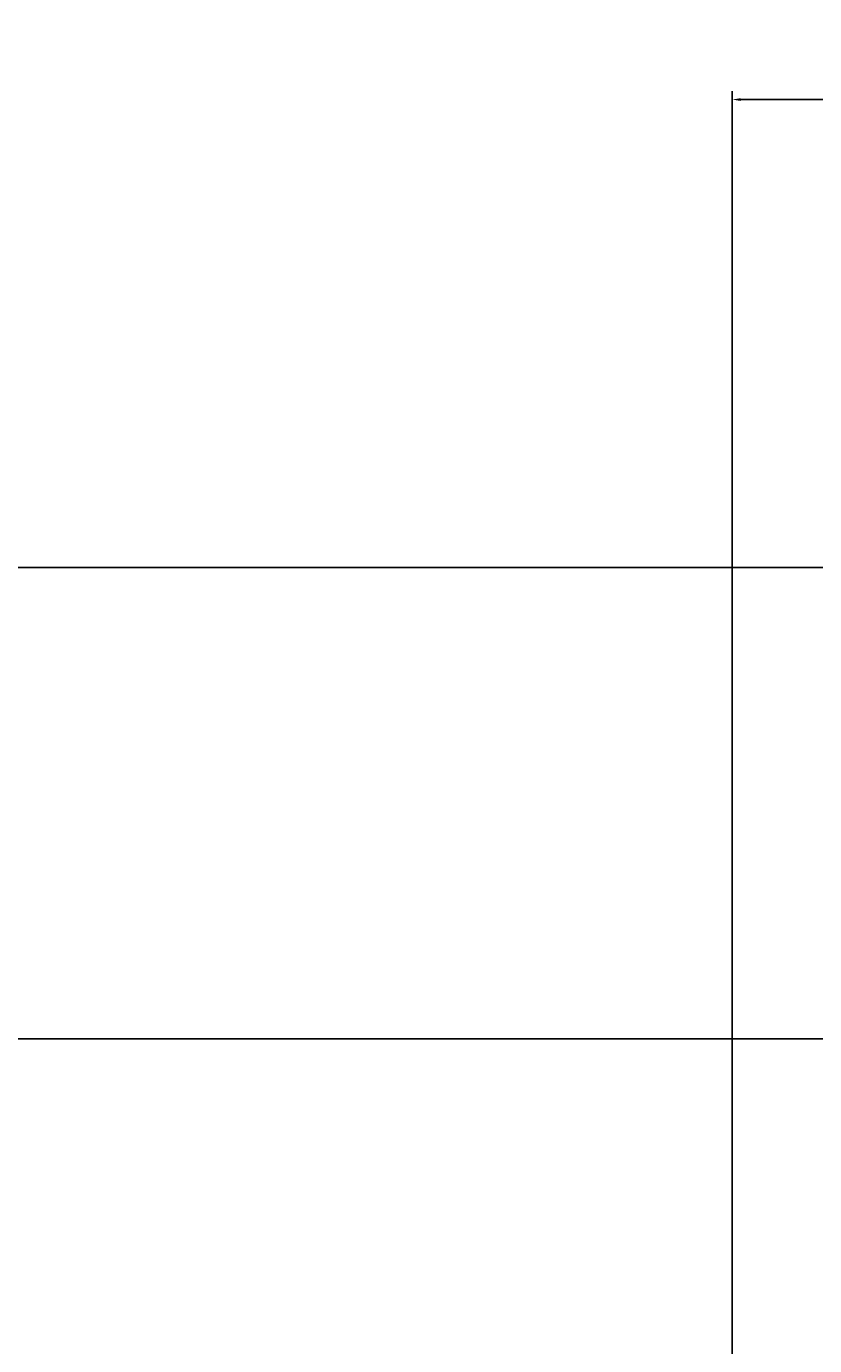
# Model space of a CAD drawing. Units: millimetres. Extents: x -53 to 92, y -147 to 37.
# Tile 14 of 16: x -6 to 11, y 9 to 37. Entities that reach past the tile are written whole.
import ezdxf

# ---------------------------------------------------------------- set-up
doc = ezdxf.new("R2010")
doc.units = ezdxf.units.MM
doc.header["$MEASUREMENT"] = 0
doc.layers.add('M-DIMS', color=2, linetype='Continuous', lineweight=25)
doc.styles.get("Standard").update_dxf_attribs({"font": 'arial.ttf'})
doc.dimstyles.get("Standard").update_dxf_attribs({"dimtxt": 0.18, "dimasz": 0.18, "dimexe": 0.18, "dimexo": 0.0625, "dimgap": 0.09, "dimtad": 0, "dimtih": 1, "dimtoh": 1, "dimdec": 4, "dimzin": 0, "dimdsep": 46, "dimtxsty": 'Standard', "dimcen": 0.09, "dimadec": 0, "dimazin": 0, "dimtfac": 1, "dimtdec": 4, "dimtofl": 0, "dimtmove": 0, "dimatfit": 3, "dimfxl": 1, "dimtolj": 1, "dimtzin": 0, "dimarcsym": 0})

# ---------------------------------------------------------------- blocks, each defined once
blk = doc.blocks.new('*D5')
at = {"layer": 'Defpoints', "color": 0, "transparency": 16777216}
for p in [(28.602, 35.845), (28.602, 15.91), (9.265, -3.88)]:
    blk.add_point(p, dxfattribs=at)
at = {"layer": 'M-DIMS', "color": 0, "lineweight": -2, "transparency": 16777216}
for p, q in [((9.265, -3.817), (9.265, 36.025)), ((9.445, 35.845), (16.674, 35.845)), ((28.422, 35.845), (21.192, 35.845)), ((28.602, 15.973), (28.602, 36.025))]:
    blk.add_line(p, q, dxfattribs=at)
at = {"layer": 'M-DIMS', "color": 0, "transparency": 16777216}
for points in [[(9.445, 35.875), (9.445, 35.815), (9.265, 35.845)], [(28.422, 35.875), (28.422, 35.815), (28.602, 35.845)]]:
    blk.add_solid(points, dxfattribs=at)
at = {"layer": 'M-DIMS', "color": 0, "transparency": 16777216, "insert": (18.933, 35.845), "char_height": 0.18, "attachment_point": 5}
blk.add_mtext('\\A1;{\\H16.66667x;20}', dxfattribs=at)
blk = doc.blocks.new('*D6')
at = {"layer": 'Defpoints', "color": 0, "transparency": 16777216}
for p in [(-26.95, 15.91), (28.602, 15.91), (9.355, -3.79)]:
    blk.add_point(p, dxfattribs=at)
at = {"layer": 'M-DIMS', "color": 0, "lineweight": -2, "transparency": 16777216}
for p, q in [((28.539, 15.91), (-27.13, 15.91)), ((-26.95, 15.73), (-26.95, 7.682)), ((-26.95, -3.61), (-26.95, 4.438)), ((9.292, -3.79), (-27.13, -3.79))]:
    blk.add_line(p, q, dxfattribs=at)
at = {"layer": 'M-DIMS', "color": 0, "transparency": 16777216}
for points in [[(-26.98, 15.73), (-26.92, 15.73), (-26.95, 15.91)], [(-26.98, -3.61), (-26.92, -3.61), (-26.95, -3.79)]]:
    blk.add_solid(points, dxfattribs=at)
at = {"layer": 'M-DIMS', "color": 0, "transparency": 16777216, "insert": (-26.95, 6.06), "char_height": 0.18, "attachment_point": 5}
blk.add_mtext('\\A1;{\\H16.66667x;20}', dxfattribs=at)
blk = doc.blocks.new('*D17')
at = {"layer": 'Defpoints', "color": 0, "transparency": 16777216}
for p in [(-46.81, 25.909), (28.564, 25.909), (18.165, -111.975)]:
    blk.add_point(p, dxfattribs=at)
at = {"layer": 'M-DIMS', "color": 0, "lineweight": -2, "transparency": 16777216}
for p, q in [((28.502, 25.909), (-46.99, 25.909)), ((-46.81, 25.729), (-46.81, -42.851)), ((-46.81, -111.795), (-46.81, -43.215)), ((18.102, -111.975), (-46.99, -111.975))]:
    blk.add_line(p, q, dxfattribs=at)
at = {"layer": 'M-DIMS', "color": 0, "transparency": 16777216}
for points in [[(-46.84, 25.729), (-46.78, 25.729), (-46.81, 25.909)], [(-46.84, -111.795), (-46.78, -111.795), (-46.81, -111.975)]]:
    blk.add_solid(points, dxfattribs=at)
at = {"layer": 'M-DIMS', "color": 0, "transparency": 16777216, "insert": (-46.81, -43.033), "char_height": 0.18, "attachment_point": 5}
blk.add_mtext('\\A1;137.88', dxfattribs=at)

msp = doc.modelspace()

# ---------------------------------------------------------------- dimensions: what is measured, and where the dimension line sits
at = {"layer": 'M-DIMS'}
dim = msp.add_linear_dim(base=(28.60189, 35.84496), p1=(9.26461, -3.87977), p2=(28.60189, 15.91006), text='{\\H16.66667x;20}', dimstyle='Standard', override={"dimclrd": 0, "dimclre": 0, "dimclrt": 0}, dxfattribs=at)
dim.commit()
dim.dimension.update_dxf_attribs({"geometry": '*D5', "text_midpoint": (18.93325, 35.84496)})
dim = msp.add_linear_dim(base=(-46.8103, 25.90924), p1=(18.16452, -111.97467), p2=(28.56407, 25.90924), angle=90, dimstyle='Standard', override={"dimdec": 2, "dimlfac": 1, "dimrnd": 0, "dimzin": 0, "dimdsep": 46, "dimlunit": 2}, dxfattribs=at)
dim.commit()
dim.dimension.update_dxf_attribs({"geometry": '*D17', "text_midpoint": (-46.8103, -43.03271)})
dim = msp.add_linear_dim(base=(-26.95014, 15.91006), p1=(9.35461, -3.78977), p2=(28.60189, 15.91006), angle=90, text='{\\H16.66667x;20}', dimstyle='Standard', override={"dimclrd": 0, "dimclre": 0, "dimclrt": 0}, dxfattribs=at)
dim.commit()
dim.dimension.update_dxf_attribs({"geometry": '*D6', "text_midpoint": (-26.95014, 6.06014)})

doc.saveas('drawing.dxf')
